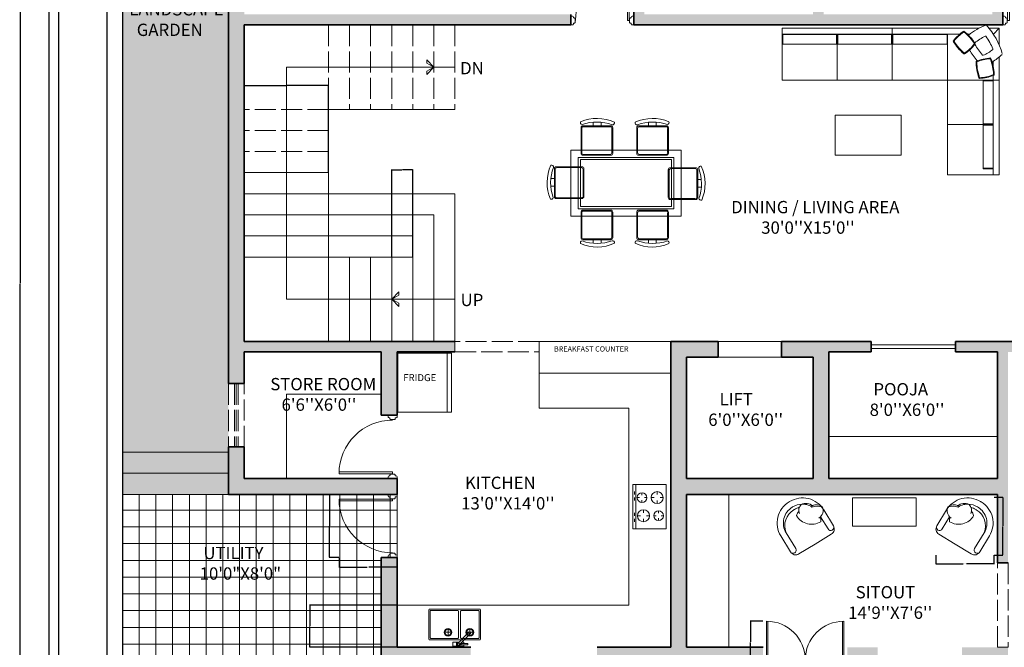
# Model space of a CAD drawing. Units: inches. Extents: x 84 to 1044, y -280 to 906.
# Tile 49 of 105: x 84 to 645, y 160 to 517. Entities that reach past the tile are written whole.
import ezdxf

# ---------------------------------------------------------------- set-up
doc = ezdxf.new("R2010")
doc.units = ezdxf.units.IN
doc.linetypes.add('ACAD_ISO02W100', pattern=[15, 12, -3])
for name, color, linetype, lineweight in [('00 FURNITURE', 15, 'Continuous', 15), ('A-ANNO-DIMS', 2, 'Continuous', 18), ('A-ANNO-SYMB', 7, 'Continuous', 15), ('A-ANNO-TEXT', 7, 'Continuous', 13), ('A-ANNO-TTLB', 7, 'Continuous', 25), ('A-AREA-IDEN', 7, 'Continuous', 13), ('A-DOOR', 4, 'Continuous', 18), ('A-EQPM', 8, 'Continuous', 15), ('A-FLOR-CASE', 8, 'Continuous', 18), ('A-FLOR-FIXT', 9, 'Continuous', 15), ('A-FLOR-STRS-OVHD', 144, 'ACAD_ISO02W100', 13), ('A-FURN', 8, 'Continuous', 15), ('A-GLAZ-HIGH', 160, 'ACAD_ISO02W100', 13), ('A-STAIRCASE', 144, 'Continuous', 18), ('A-WALL-OVHD', 8, 'ACAD_ISO02W100', 13), ('C-PROP', 7, 'Continuous', 25), ('L-HRDS', 32, 'Continuous', 18), ('WALL', 250, 'Continuous', 35), ('WINDOW', 160, 'Continuous', 13)]:
    doc.layers.add(name, color=color, linetype=linetype, lineweight=lineweight)
for name, color, linetype, lineweight, true_color in [('A-FLOR-PATT', 251, 'Continuous', 9, 0x705861), ('A-FLOR-STRS-PATT', 35, 'Continuous', 9, 0x947764), ('A-WALL-PATT', 251, 'Continuous', 9, 0x636466), ('L-PLNT-PATT', 9, 'Continuous', 9, 0xafd9aa)]:
    doc.layers.add(name, color=color, linetype=linetype, lineweight=lineweight, true_color=true_color)
doc.styles.add('1-100DIM', font='txt', dxfattribs={"height": 0.3})
doc.styles.get("Standard").update_dxf_attribs({"font": 'arial.ttf'})
doc.dimstyles.get("Standard").update_dxf_attribs({"dimtxt": 0.18, "dimasz": 0.18, "dimexe": 0.18, "dimexo": 0.0625, "dimgap": 0.09, "dimtad": 0, "dimtih": 1, "dimtoh": 1, "dimdec": 4, "dimzin": 0, "dimdsep": 46, "dimtxsty": 'Standard', "dimcen": 0.09, "dimadec": 0, "dimazin": 0, "dimtfac": 1, "dimtdec": 4, "dimtofl": 0, "dimtmove": 0, "dimatfit": 3, "dimfxl": 1, "dimtolj": 1, "dimtzin": 0, "dimarcsym": 0})

# ---------------------------------------------------------------- blocks, each defined once
blk = doc.blocks.new('PUJA')
at = {"layer": '00 FURNITURE'}
for p, q in [((-1940.35, -16093.35), (-1958.14, -16093.35)), ((-1940.35, -16093.93), (-1958.13, -16093.93)), ((-1941.8, -16091.75), (-1938.89, -16091.75)), ((-1941.8, -16092.33), (-1941.8, -16091.75)), ((-1941.22, -16092.62), (-1941.51, -16092.62)), ((-1940.35, -16093.35), (-1940.35, -16093.93)), ((-1939.18, -16092.62), (-1939.47, -16092.62)), ((-1938.89, -16091.75), (-1938.89, -16092.33)), ((-1940.35, -16128.93), (-1958.14, -16128.93)), ((-1940.35, -16128.35), (-1958.13, -16128.35)), ((-1941.8, -16129.96), (-1941.8, -16130.54)), ((-1941.8, -16130.54), (-1938.89, -16130.54)), ((-1941.22, -16129.66), (-1941.51, -16129.66)), ((-1940.35, -16128.93), (-1940.35, -16128.35)), ((-1939.18, -16129.66), (-1939.47, -16129.66)), ((-1938.89, -16130.54), (-1938.89, -16129.96))]:
    blk.add_line(p, q, dxfattribs=at)
for points in [[(-1939.47, -16092.62), (-1939.47, -16092.91, -0.414214), (-1939.76, -16093.21), (-1940.93, -16093.21, -0.414214), (-1941.22, -16092.91), (-1941.22, -16092.62)], [(-1939.47, -16129.66), (-1939.47, -16129.37, 0.414214), (-1939.76, -16129.08), (-1940.93, -16129.08, 0.414214), (-1941.22, -16129.37), (-1941.22, -16129.66)]]:
    blk.add_lwpolyline(points, format="xyb", dxfattribs=at)
for centre, radius, start, end in [((-1940.35, -16093.35), 17.79, 180, 270), ((-1941.51, -16092.33), 0.292, 180, 270), ((-1939.18, -16092.33), 0.292, 270, 0), ((-1940.35, -16128.93), 17.79, 90, 180), ((-1941.51, -16129.96), 0.292, 90, 180), ((-1939.18, -16129.96), 0.292, 0, 90)]:
    blk.add_arc(centre, radius, start, end, dxfattribs=at)
blk = doc.blocks.new('DDD')
at = {"layer": '00 FURNITURE'}
for p, q in [((-12579.77, -15859.53), (-12579.77, -15829.05)), ((-12578.77, -15859.53), (-12578.77, -15829.03)), ((-12612.02, -15857.03), (-12612.02, -15862.03)), ((-12611.02, -15857.03), (-12612.02, -15857.03)), ((-12610.52, -15858.03), (-12610.52, -15857.53)), ((-12577.52, -15858.03), (-12577.52, -15857.53)), ((-12577.02, -15857.03), (-12576.02, -15857.03)), ((-12576.02, -15857.03), (-12576.02, -15862.03)), ((-12612.02, -15862.03), (-12611.02, -15862.03)), ((-12610.52, -15861.53), (-12610.52, -15861.03)), ((-12578.77, -15859.53), (-12579.77, -15859.53)), ((-12577.52, -15861.53), (-12577.52, -15861.03)), ((-12576.02, -15862.03), (-12577.02, -15862.03))]:
    blk.add_line(p, q, dxfattribs=at)
for points in [[(-12610.52, -15861.03), (-12610.02, -15861.03, 0.414214), (-12609.52, -15860.53), (-12609.52, -15858.53, 0.414214), (-12610.02, -15858.03), (-12610.52, -15858.03)], [(-12577.52, -15861.03), (-12578.02, -15861.03, -0.414214), (-12578.52, -15860.53), (-12578.52, -15858.53, -0.414214), (-12578.02, -15858.03), (-12577.52, -15858.03)]]:
    blk.add_lwpolyline(points, format="xyb", dxfattribs=at)
for centre, radius, start, end in [((-12578.77, -15859.53), 30.5, 90, 180), ((-12611.02, -15857.53), 0.5, 0, 90), ((-12577.02, -15857.53), 0.5, 90, 180), ((-12611.02, -15861.53), 0.5, 270, 0), ((-12577.02, -15861.53), 0.5, 180, 270)]:
    blk.add_arc(centre, radius, start, end, dxfattribs=at)
blk = doc.blocks.new('CHAIR-LOUNGE')
for points in [[(10.9, 6.11), (20.11, 0.51, 0.414214), (24.96, 1.7), (30.46, 10.75, 0.414214), (25.72, 30.16), (25.57, 30.25), (25.42, 30.34, 0.414214), (6.01, 25.61), (0.51, 16.55, 0.414214), (1.69, 11.7), (10.9, 6.11)], [(8.7, 20.85, -0.356772), (6.69, 27.28, -0.249542), (12.51, 28.04, 9.61688)], [(6.69, 27.28, -0.14773), (12.68, 27.2, -0.213343), (18.88, 28.63, -0.178662)], [(12.19, 27.77, -0.306663), (18.88, 28.63, -0.30633), (19.83, 23.56, 0.872847)], [(18.37, 28.86, -0.130591), (23.59, 27.33), (23.74, 27.24)], [(8, 21.4, 0.165541), (7.72, 18.84, 0.425989), (21.45, 22.34, 0.121523), (20.16, 24.75, -7.115464)], [(19.9, 27.06, -0.072384), (22.67, 25.82), (22.82, 25.73)], [(27.44, 12.59, 0.372719), (22.97, 25.63), (22.82, 25.73)], [(27.44, 12.59, 0.414214), (23.89, 27.14), (23.74, 27.24)], [(7.74, 21.66), (3.53, 14.72, -0.414214), (1.1, 14.13), (1.1, 14.13, -0.414214), (0.51, 16.55)], [(27.44, 12.59), (21.94, 3.53, 0.414214), (22.53, 1.11), (22.53, 1.11, 0.414214), (24.96, 1.7)]]:
    blk.add_lwpolyline(points, format="xyb")
blk = doc.blocks.new('WIN-HIGH-36IN')
for p, q in [((3.5, 36), (3.5, 0)), ((4.5, 36), (4.5, 0)), ((5.5, 36), (5.5, 0))]:
    blk.add_line(p, q)
blk.add_lwpolyline([(0, 0), (9, 0), (9, 36), (0, 36)], close=True)
blk = doc.blocks.new('STAIR-DIRECTION-HEAD')
for p, q in [((0, 4.1), (4.1, 8.21)), ((4.1, 6.33), (0, 4.1)), ((4.1, 8.21), (4.1, 6.33)), ((0, 4.1), (4.1, -0.01)), ((4.1, 1.87), (0, 4.1)), ((4.1, -0.01), (4.1, 1.87))]:
    blk.add_line(p, q)
blk = doc.blocks.new('*D38')
at = {"layer": 'A-ANNO-DIMS', "color": 0, "lineweight": -2, "transparency": 16777216}
for p, q in [((266.12, 247.12), (260.6, 247.12)), ((260.78, 246.94), (260.78, 229.3)), ((260.78, 211.3), (260.78, 228.94)), ((266.12, 211.12), (260.6, 211.12))]:
    blk.add_line(p, q, dxfattribs=at)
at = {"layer": 'A-ANNO-DIMS', "color": 0, "transparency": 16777216}
for points in [[(260.75, 246.94), (260.81, 246.94), (260.78, 247.12)], [(260.75, 211.3), (260.81, 211.3), (260.78, 211.12)]]:
    blk.add_solid(points, dxfattribs=at)
at = {"layer": 'Defpoints', "color": 0, "transparency": 16777216}
for p in [(260.78, 247.12), (266.18, 247.12), (266.18, 211.12)]:
    blk.add_point(p, dxfattribs=at)
at = {"layer": 'A-ANNO-DIMS', "color": 0, "transparency": 16777216, "insert": (260.78, 229.12), "char_height": 0.18, "attachment_point": 5}
blk.add_mtext('\\A1;DOOR 36 TYP.', dxfattribs=at)
blk = doc.blocks.new('*D39')
at = {"layer": 'A-ANNO-DIMS', "color": 0, "lineweight": -2, "transparency": 16777216}
for p, q in [((266.18, 211.06), (266.18, 205.54)), ((299.18, 211.06), (299.18, 205.54)), ((266.36, 205.72), (282.15, 205.72)), ((299, 205.72), (283.21, 205.72))]:
    blk.add_line(p, q, dxfattribs=at)
at = {"layer": 'A-ANNO-DIMS', "color": 0, "transparency": 16777216}
for points in [[(266.36, 205.75), (266.36, 205.69), (266.18, 205.72)], [(299, 205.75), (299, 205.69), (299.18, 205.72)]]:
    blk.add_solid(points, dxfattribs=at)
at = {"layer": 'Defpoints', "color": 0, "transparency": 16777216}
for p in [(266.18, 211.12), (299.18, 211.12), (266.18, 205.72)]:
    blk.add_point(p, dxfattribs=at)
at = {"layer": 'A-ANNO-DIMS', "color": 0, "transparency": 16777216, "insert": (282.68, 205.72), "char_height": 0.18, "attachment_point": 5}
blk.add_mtext('\\A1;33 TYP.', dxfattribs=at)
blk = doc.blocks.new('*D43')
at = {"layer": 'A-ANNO-DIMS', "color": 0, "lineweight": -2, "transparency": 16777216}
for p, q in [((507.51, 174.94), (500.19, 174.94)), ((500.37, 174.76), (500.37, 163.21)), ((500.37, 151.3), (500.37, 162.85)), ((507.51, 151.12), (500.19, 151.12))]:
    blk.add_line(p, q, dxfattribs=at)
at = {"layer": 'A-ANNO-DIMS', "color": 0, "transparency": 16777216}
for points in [[(500.34, 174.76), (500.4, 174.76), (500.37, 174.94)], [(500.34, 151.3), (500.4, 151.3), (500.37, 151.12)]]:
    blk.add_solid(points, dxfattribs=at)
at = {"layer": 'Defpoints', "color": 0, "transparency": 16777216}
for p in [(507.57, 174.94), (500.37, 151.12), (507.57, 151.12)]:
    blk.add_point(p, dxfattribs=at)
at = {"layer": 'A-ANNO-DIMS', "color": 0, "transparency": 16777216, "insert": (500.37, 163.03), "char_height": 0.18, "attachment_point": 5}
blk.add_mtext('\\A1;24', dxfattribs=at)
blk = doc.blocks.new('*D58')
at = {"layer": 'A-ANNO-DIMS', "color": 0, "lineweight": -2, "transparency": 16777216}
for p, q in [((605.9, 212.52), (605.9, 207.43)), ((606.08, 207.61), (621.5, 207.61)), ((638.84, 207.61), (623.41, 207.61)), ((639.02, 212.52), (639.02, 207.43))]:
    blk.add_line(p, q, dxfattribs=at)
at = {"layer": 'A-ANNO-DIMS', "color": 0, "transparency": 16777216}
for points in [[(606.08, 207.64), (606.08, 207.58), (605.9, 207.61)], [(638.84, 207.64), (638.84, 207.58), (639.02, 207.61)]]:
    blk.add_solid(points, dxfattribs=at)
at = {"layer": 'Defpoints', "color": 0, "transparency": 16777216}
for p in [(605.9, 212.58), (639.02, 212.58), (639.02, 207.61)]:
    blk.add_point(p, dxfattribs=at)
at = {"layer": 'A-ANNO-DIMS', "color": 0, "transparency": 16777216, "insert": (622.46, 207.61), "char_height": 0.18, "attachment_point": 5}
blk.add_mtext('\\A1;CHAIR 33 TYP.', dxfattribs=at)
blk = doc.blocks.new('*D59')
at = {"layer": 'A-ANNO-DIMS', "color": 0, "lineweight": -2, "transparency": 16777216}
for p, q in [((639.08, 245.58), (644.17, 245.58)), ((643.99, 245.4), (643.99, 229.26)), ((643.99, 212.76), (643.99, 228.9)), ((639.08, 212.58), (644.17, 212.58))]:
    blk.add_line(p, q, dxfattribs=at)
at = {"layer": 'A-ANNO-DIMS', "color": 0, "transparency": 16777216}
for points in [[(643.96, 245.4), (644.02, 245.4), (643.99, 245.58)], [(643.96, 212.76), (644.02, 212.76), (643.99, 212.58)]]:
    blk.add_solid(points, dxfattribs=at)
at = {"layer": 'Defpoints', "color": 0, "transparency": 16777216}
for p in [(639.02, 245.58), (643.99, 245.58), (639.02, 212.58)]:
    blk.add_point(p, dxfattribs=at)
at = {"layer": 'A-ANNO-DIMS', "color": 0, "transparency": 16777216, "insert": (643.99, 229.08), "char_height": 0.18, "attachment_point": 5}
blk.add_mtext('\\A1;33 TYP.', dxfattribs=at)
blk = doc.blocks.new('*D61')
at = {"layer": 'A-ANNO-DIMS', "color": 0, "lineweight": -2, "transparency": 16777216}
for p, q in [((134.12, 856.12), (84.4, 856.12)), ((84.58, 855.94), (84.58, 367.3)), ((84.58, -121.7), (84.58, 366.94)), ((134.12, -121.88), (84.4, -121.88))]:
    blk.add_line(p, q, dxfattribs=at)
at = {"layer": 'A-ANNO-DIMS', "color": 0, "transparency": 16777216}
for points in [[(84.55, 855.94), (84.61, 855.94), (84.58, 856.12)], [(84.55, -121.7), (84.61, -121.7), (84.58, -121.88)]]:
    blk.add_solid(points, dxfattribs=at)
at = {"layer": 'Defpoints', "color": 0, "transparency": 16777216}
for p in [(84.58, 856.12), (134.18, 856.12), (134.18, -121.88)]:
    blk.add_point(p, dxfattribs=at)
at = {"layer": 'A-ANNO-DIMS', "color": 0, "transparency": 16777216, "insert": (84.58, 367.12), "char_height": 0.18, "attachment_point": 5}
blk.add_mtext('\\A1;978', dxfattribs=at)
blk = doc.blocks.new('*D62')
at = {"layer": 'A-ANNO-DIMS', "color": 0, "lineweight": -2, "transparency": 16777216}
for p, q in [((203.18, 709.18), (203.18, 905.9)), ((203.36, 905.72), (549.23, 905.72)), ((895.89, 905.72), (550.02, 905.72)), ((896.07, 400.18), (896.07, 905.9))]:
    blk.add_line(p, q, dxfattribs=at)
at = {"layer": 'A-ANNO-DIMS', "color": 0, "transparency": 16777216}
for points in [[(203.36, 905.75), (203.36, 905.69), (203.18, 905.72)], [(895.89, 905.75), (895.89, 905.69), (896.07, 905.72)]]:
    blk.add_solid(points, dxfattribs=at)
at = {"layer": 'Defpoints', "color": 0, "transparency": 16777216}
for p in [(896.07, 905.72), (203.18, 709.12), (896.07, 400.12)]:
    blk.add_point(p, dxfattribs=at)
at = {"layer": 'A-ANNO-DIMS', "color": 0, "transparency": 16777216, "insert": (549.63, 905.72), "char_height": 0.18, "attachment_point": 5}
blk.add_mtext('\\A1;692.9', dxfattribs=at)
blk = doc.blocks.new('*D71')
at = {"layer": 'A-ANNO-DIMS', "color": 0, "lineweight": -2, "transparency": 16777216}
for p, q in [((212.18, 430.18), (212.18, 479.9)), ((212.36, 479.72), (235.96, 479.72)), ((260, 479.72), (236.4, 479.72)), ((260.18, 430.18), (260.18, 479.9))]:
    blk.add_line(p, q, dxfattribs=at)
at = {"layer": 'A-ANNO-DIMS', "color": 0, "transparency": 16777216}
for points in [[(212.36, 479.75), (212.36, 479.69), (212.18, 479.72)], [(260, 479.75), (260, 479.69), (260.18, 479.72)]]:
    blk.add_solid(points, dxfattribs=at)
at = {"layer": 'Defpoints', "color": 0, "transparency": 16777216}
for p in [(260.18, 479.72), (212.18, 430.12), (260.18, 430.12)]:
    blk.add_point(p, dxfattribs=at)
at = {"layer": 'A-ANNO-DIMS', "color": 0, "transparency": 16777216, "insert": (236.18, 479.72), "char_height": 0.18, "attachment_point": 5}
blk.add_mtext('\\A1;48', dxfattribs=at)
blk = doc.blocks.new('*D72')
at = {"layer": 'A-ANNO-DIMS', "color": 0, "lineweight": -2, "transparency": 16777216}
for p, q in [((296.18, 382.18), (296.18, 431.9)), ((296.36, 431.72), (301.97, 431.72)), ((308, 431.72), (302.39, 431.72)), ((308.18, 382.18), (308.18, 431.9))]:
    blk.add_line(p, q, dxfattribs=at)
at = {"layer": 'A-ANNO-DIMS', "color": 0, "transparency": 16777216}
for points in [[(296.36, 431.75), (296.36, 431.69), (296.18, 431.72)], [(308, 431.75), (308, 431.69), (308.18, 431.72)]]:
    blk.add_solid(points, dxfattribs=at)
at = {"layer": 'Defpoints', "color": 0, "transparency": 16777216}
for p in [(308.18, 431.72), (296.18, 382.12), (308.18, 382.12)]:
    blk.add_point(p, dxfattribs=at)
at = {"layer": 'A-ANNO-DIMS', "color": 0, "transparency": 16777216, "insert": (302.18, 431.72), "char_height": 0.18, "attachment_point": 5}
blk.add_mtext('\\A1;12', dxfattribs=at)
blk = doc.blocks.new('*D79')
at = {"layer": 'A-ANNO-DIMS', "color": 0, "lineweight": -2, "transparency": 16777216}
for p, q in [((299.12, 184.12), (249.4, 184.12)), ((249.58, 183.94), (249.58, 172.3)), ((249.58, 160.3), (249.58, 171.94)), ((299.12, 160.12), (249.4, 160.12))]:
    blk.add_line(p, q, dxfattribs=at)
at = {"layer": 'A-ANNO-DIMS', "color": 0, "transparency": 16777216}
for points in [[(249.55, 183.94), (249.61, 183.94), (249.58, 184.12)], [(249.55, 160.3), (249.61, 160.3), (249.58, 160.12)]]:
    blk.add_solid(points, dxfattribs=at)
at = {"layer": 'Defpoints', "color": 0, "transparency": 16777216}
for p in [(249.58, 184.12), (299.18, 184.12), (299.18, 160.12)]:
    blk.add_point(p, dxfattribs=at)
at = {"layer": 'A-ANNO-DIMS', "color": 0, "transparency": 16777216, "insert": (249.58, 172.12), "char_height": 0.18, "attachment_point": 5}
blk.add_mtext('\\A1;24', dxfattribs=at)

msp = doc.modelspace()

# ---------------------------------------------------------------- hatches: boundary and pattern name
at = {"layer": 'A-FLOR-PATT', "transparency": 33554597}
h = msp.add_hatch(dxfattribs=at)
h.set_pattern_fill('ANSI37', color=256, scale=3, angle=45)
h.paths.add_polyline_path([(290.179, 211.12), (299.179, 211.12), (299.179, 247.12), (203.179, 247.12), (143.179, 247.12), (143.179, 151.12), (203.179, 151.12), (203.179, 155.12), (290.179, 155.12)])
at = {"layer": 'A-FLOR-STRS-PATT', "transparency": 33554567}
h = msp.add_hatch(color=256, dxfattribs=at)
h.dxf.hatch_style = 1
h.paths.add_polyline_path([(650.074, 91.12), (638.074, 91.12), (638.074, 67.12), (455.074, 67.12), (455.074, 55.12), (650.074, 55.12)], flags=17)
h.paths.add_polyline_path([(662.074, 91.12), (650.074, 91.12), (650.074, 55.12), (455.074, 55.12), (455.074, 43.12), (662.074, 43.12)])
h.paths.add_polyline_path([(674.074, 91.12), (671.074, 91.12), (662.074, 91.12), (662.074, 43.12), (455.074, 43.12), (455.074, 31.12), (674.074, 31.12)])
h.paths.add_polyline_path([(227.179, 151.12), (203.179, 151.12), (143.179, 151.12), (143.179, 139.12), (227.179, 139.12)])
h.paths.add_polyline_path([(227.179, 139.12), (143.179, 139.12), (143.179, 127.12), (227.179, 127.12)])
h.paths.add_polyline_path([(203.179, 271.12), (143.179, 271.12), (143.179, 259.12), (203.179, 259.12)])
h.paths.add_polyline_path([(203.179, 259.12), (143.179, 259.12), (143.179, 247.12), (203.179, 247.12)])
h.paths.add_polyline_path([(203.179, 769.12), (143.179, 769.12), (143.179, 757.12), (203.179, 757.12)])
h.paths.add_polyline_path([(203.179, 757.12), (143.179, 757.12), (143.179, 745.12), (203.179, 745.12)])
h.paths.add_polyline_path([(434.074, 847.12), (422.074, 847.12), (422.074, 769.12), (434.074, 769.12)])
h.paths.add_polyline_path([(422.074, 847.12), (410.074, 847.12), (410.074, 769.12), (422.074, 769.12)])
at = {"layer": 'A-WALL-PATT', "transparency": 33554597}
h = msp.add_hatch(color=256, dxfattribs=at)
h.dxf.hatch_style = 1
h.paths.add_polyline_path([(671.074, 100.12), (647.074, 100.12), (647.074, 160.12), (641.074, 160.12), (620.824, 160.12), (620.824, 151.12), (638.074, 151.12), (638.074, 91.12), (671.074, 91.12)])
h.paths.add_polyline_path([(791.074, 100.12), (743.074, 100.12), (743.074, 91.12), (791.074, 91.12)])
h.paths.add_polyline_path([(896.074, 346.12), (887.074, 346.12), (887.074, 334.12), (870.955, 334.12), (833.074, 334.12), (804.574, 334.12), (804.574, 328.12), (887.074, 328.12), (887.074, 100.12), (863.074, 100.12), (863.074, 91.12), (896.074, 91.12)])
h.paths.add_polyline_path([(507.574, 154.729), (507.574, 160.12), (464.074, 160.12), (464.074, 247.12), (641.074, 247.12), (641.074, 208.12), (647.074, 208.12), (647.074, 328.12), (659.074, 328.12), (659.074, 334.12), (617.074, 334.12), (617.074, 328.12), (641.074, 328.12), (641.074, 256.12), (545.074, 256.12), (545.074, 328.12), (569.074, 328.12), (569.074, 334.12), (518.074, 334.12), (518.074, 325.12), (536.074, 325.12), (536.074, 256.12), (464.074, 256.12), (464.074, 325.12), (482.074, 325.12), (482.074, 334.12), (455.074, 334.12), (455.074, 160.12), (413.127, 160.12), (413.127, 151.12), (455.074, 151.12), (455.074, 91.12), (464.074, 91.12), (464.074, 151.12), (507.574, 151.12)])
h.paths.add_polyline_path([(572.824, 160.12), (555.574, 160.12), (555.574, 151.12), (572.824, 151.12)], flags=17)
h.paths.add_polyline_path([(341.127, 160.12), (299.179, 160.12), (299.179, 211.12), (294.179, 211.12), (290.179, 211.12), (290.179, 151.12), (341.127, 151.12)])
h.paths.add_polyline_path([(299.179, 256.12), (212.179, 256.12), (212.179, 274.12), (203.179, 274.12), (203.179, 247.12), (299.179, 247.12)])
h.paths.add_polyline_path([(212.179, 514.12), (398.074, 514.12), (398.074, 519.12), (398.074, 520.12), (212.179, 520.12), (212.179, 574.12), (203.179, 574.12), (203.179, 310.12), (212.179, 310.12), (212.179, 328.12), (290.179, 328.12), (290.179, 292.12), (299.179, 292.12), (299.179, 328.12), (332.179, 328.12), (332.179, 334.12), (212.179, 334.12)])
h.paths.add_polyline_path([(287.127, 709.12), (203.179, 709.12), (203.179, 646.12), (212.179, 646.12), (212.179, 700.12), (287.127, 700.12)])
h.paths.add_polyline_path([(470.074, 709.12), (359.127, 709.12), (359.127, 700.12), (434.074, 700.12), (434.074, 574.12), (440.074, 574.12), (440.074, 622.12), (464.074, 622.12), (464.074, 628.12), (440.074, 628.12), (440.074, 700.12), (470.074, 700.12)])
h.paths.add_polyline_path([(572.074, 709.12), (506.074, 709.12), (506.074, 700.12), (536.074, 700.12), (536.074, 628.12), (494.074, 628.12), (494.074, 622.12), (536.074, 622.12), (536.074, 520.12), (440.074, 520.12), (440.074, 544.12), (434.074, 544.12), (434.074, 514.12), (644.074, 514.12), (644.074, 519.12), (644.074, 544.12), (638.074, 544.12), (638.074, 520.12), (542.074, 520.12), (542.074, 622.12), (584.074, 622.12), (584.074, 628.12), (542.074, 628.12), (542.074, 700.12), (572.074, 700.12)])
h.paths.add_polyline_path([(698.074, 709.12), (608.074, 709.12), (608.074, 700.12), (638.074, 700.12), (638.074, 628.12), (614.074, 628.12), (614.074, 622.12), (638.074, 622.12), (638.074, 574.12), (644.074, 574.12), (644.074, 700.12), (698.074, 700.12)])
h.paths.add_polyline_path([(833.074, 709.12), (770.074, 709.12), (770.074, 700.12), (824.074, 700.12), (824.074, 646.12), (833.074, 646.12)])
h.paths.add_polyline_path([(833.074, 574.12), (824.074, 574.12), (824.074, 520.12), (791.244, 520.12), (712.904, 520.12), (680.074, 520.12), (680.074, 514.12), (695.074, 514.12), (695.074, 491.62), (704.074, 491.62), (704.074, 511.12), (833.074, 511.12)])
h.paths.add_polyline_path([(704.074, 419.62), (695.074, 419.62), (695.074, 370.12), (704.074, 370.12)])
h.paths.add_polyline_path([(896.074, 400.12), (833.074, 400.12), (833.074, 364.12), (839.074, 364.12), (839.074, 394.12), (887.074, 394.12), (887.074, 382.12), (896.074, 382.12)])
h.paths.add_polyline_path([(732.574, 334.12), (695.074, 334.12), (695.074, 328.12), (732.574, 328.12)])
at = {"layer": 'L-PLNT-PATT', "transparency": 33554597}
h = msp.add_hatch(color=256, dxfattribs=at)
h.dxf.hatch_style = 1
h.paths.add_polyline_path([(434.074, 769.12), (386.074, 769.12), (386.074, 709.12), (434.074, 709.12)])
h.paths.add_polyline_path([(896.074, 847.12), (434.074, 847.12), (434.074, 769.12), (434.074, 709.12), (470.074, 709.12), (506.074, 709.12), (572.074, 709.12), (608.074, 709.12), (698.074, 709.12), (770.074, 709.12), (833.074, 709.12), (896.074, 709.12)])
h.paths.add_polyline_path([(983.074, 847.12), (896.074, 847.12), (896.074, 709.12), (896.074, 547.12), (932.074, 547.12), (983.074, 547.12)])
h.paths.add_polyline_path([(983.074, 547.12), (932.074, 547.12), (932.074, 265.12), (983.074, 265.12)])
h.paths.add_polyline_path([(203.179, 646.12), (203.179, 709.12), (203.179, 745.12), (143.179, 745.12), (143.179, 271.12), (203.179, 271.12), (203.179, 274.12), (203.179, 310.12), (203.179, 574.12)])

# ---------------------------------------------------------------- linework, layer by layer
at = {"layer": 'A-ANNO-SYMB'}
msp.add_lwpolyline([(332.179, 358.12), (236.179, 358.12), (236.179, 490.12), (332.179, 490.12)], dxfattribs=at)
at = {"layer": 'A-ANNO-TTLB'}
for points in [[(101.1, 905.916), (1027.308, 905.916), (1027.308, -279.764), (101.1, -279.764)], [(106.576, 900.439), (1021.832, 900.439), (1021.832, -274.288), (106.576, -274.288)]]:
    msp.add_lwpolyline(points, close=True, dxfattribs=at)
at = {"layer": 'A-DOOR'}
msp.add_line((299.179, 247.12), (299.179, 211.12), dxfattribs=at)
at = {"layer": 'A-EQPM'}
for p, q in [((482.074, 334.12), (518.074, 334.12)), ((482.074, 325.12), (518.074, 325.12)), ((433.49, 252.811), (433.49, 227.429)), ((452.402, 252.811), (433.49, 252.811)), ((435.209, 252.811), (435.209, 227.429)), ((452.402, 227.429), (452.402, 252.811)), ((434.35, 248.716), (434.35, 246.997)), ((438.648, 248.028), (438.648, 246.653)), ((447.244, 248.716), (447.244, 246.997)), ((434.35, 245.278), (434.35, 243.558)), ((435.897, 245.278), (437.272, 245.278)), ((438.648, 242.527), (438.648, 243.902)), ((441.399, 245.278), (440.023, 245.278)), ((443.805, 245.278), (445.525, 245.278)), ((447.244, 241.839), (447.244, 243.558)), ((450.682, 245.278), (448.963, 245.278)), ((434.35, 236.682), (434.35, 234.962)), ((439.507, 238.401), (439.507, 236.682)), ((448.104, 237.713), (448.104, 236.338)), ((434.35, 233.243), (434.35, 231.524)), ((436.069, 234.962), (437.788, 234.962)), ((439.507, 231.524), (439.507, 233.243)), ((442.946, 234.962), (441.227, 234.962)), ((445.353, 234.962), (446.728, 234.962)), ((448.104, 232.212), (448.104, 233.587)), ((450.854, 234.962), (449.479, 234.962)), ((433.49, 227.429), (452.402, 227.429))]:
    msp.add_line(p, q, dxfattribs=at)
for points in [[(299.707, 327.424), (327.675, 327.424), (327.675, 293.944), (299.707, 293.944)], [(327.675, 327.424), (330.111, 327.424), (330.111, 293.944), (327.675, 293.944)]]:
    msp.add_lwpolyline(points, close=True, dxfattribs=at)
for centre, major_axis, start_param, end_param in [((438.648, 245.278), (1.945, 1.945), -0.8050353, 5.47815), ((447.244, 245.278), (3.438, -0.065), 3.1674886, 9.4506739), ((439.507, 234.962), (3.438, -0.027), 3.1547976, 9.4379829), ((448.104, 234.962), (1.945, 1.945), -0.8033148, 5.4798705)]:
    msp.add_ellipse(centre, major_axis=major_axis, ratio=1, start_param=start_param, end_param=end_param, dxfattribs=at)
at = {"layer": 'A-FLOR-CASE'}
for p, q in [((455.074, 334.12), (380.179, 334.12)), ((380.179, 334.12), (380.179, 296.12)), ((455.074, 316.12), (380.179, 316.12)), ((236.179, 304.12), (236.179, 256.12)), ((290.179, 304.12), (236.179, 304.12)), ((431.074, 296.12), (380.179, 296.12)), ((431.074, 296.12), (431.074, 184.12)), ((641.074, 280.12), (545.074, 280.12)), ((488.074, 247.12), (488.074, 160.12)), ((299.179, 184.12), (431.074, 184.12))]:
    msp.add_line(p, q, dxfattribs=at)
at = {"layer": 'A-FLOR-FIXT'}
for p, q in [((317.284, 181.485), (317.284, 164.72)), ((346.27, 181.876), (317.676, 181.876)), ((318.068, 180.701), (318.068, 165.503)), ((333.736, 181.093), (318.459, 181.093)), ((334.127, 165.503), (334.127, 180.701)), ((346.662, 164.72), (346.662, 181.485)), ((325.959, 168.637), (330.464, 168.637)), ((328.212, 166.385), (328.212, 170.889)), ((338.397, 168.637), (342.901, 168.637)), ((340.329, 168.972), (339.194, 167.781)), ((340.62, 167.518), (339.761, 168.376)), ((341.215, 168.086), (340.329, 168.972)), ((340.649, 166.385), (340.649, 170.889)), ((317.676, 164.328), (346.27, 164.328)), ((318.459, 165.112), (333.736, 165.112)), ((334.413, 163), (331.033, 163)), ((331.033, 163), (331.033, 160.846)), ((333.031, 160.846), (333.031, 163)), ((333.031, 162.608), (334.021, 162.608)), ((333.751, 162.338), (339.194, 167.781)), ((340.024, 166.95), (334.582, 161.507)), ((337.222, 163), (336.075, 163)), ((337.222, 162.295), (337.222, 163)), ((340.024, 166.95), (339.194, 167.781)), ((340.024, 166.95), (341.215, 168.086)), ((331.033, 160.846), (337.222, 160.846)), ((335.185, 161.237), (333.031, 161.237)), ((335.185, 162.11), (335.185, 160.846)), ((335.655, 161.551), (335.655, 162.295)), ((335.655, 162.295), (339.415, 162.295)), ((339.415, 161.551), (335.655, 161.551)), ((337.222, 160.846), (337.222, 161.551)), ((339.415, 162.295), (339.415, 161.551))]:
    msp.add_line(p, q, dxfattribs=at)
msp.add_lwpolyline([(333.736, 181.093), (318.459, 181.093, 0.4142136), (318.068, 180.701), (318.068, 165.503, 0.4142136), (318.459, 165.112), (333.736, 165.112)], format="xyb", dxfattribs=at)
msp.add_lwpolyline([(345.487, 181.093), (335.812, 181.093, 0.4142136), (335.42, 180.701), (335.42, 165.503, 0.4142136), (335.812, 165.112), (345.487, 165.112, 0.4142136), (345.878, 165.503), (345.878, 180.701, 0.4142136)], format="xyb", close=True, dxfattribs=at)
msp.add_lwpolyline([(336.524, 165.112), (337.653, 165.112)], dxfattribs=at)
for centre, radius in [((328.212, 168.637), 2.252), ((328.212, 168.637), 1.763), ((340.649, 168.637), 2.252), ((340.649, 168.637), 1.763), ((334.166, 161.923), 0.685)]:
    msp.add_circle(centre, radius, dxfattribs=at)
for centre, radius, start, end in [((317.676, 181.485), 0.392, 90, 180), ((318.459, 180.701), 0.392, 90, 180), ((333.736, 180.701), 0.392, 0, 90), ((346.27, 181.485), 0.392, 0, 90), ((317.676, 164.72), 0.392, 180, 270), ((318.459, 165.503), 0.392, 180, 270), ((333.736, 165.503), 0.392, 270, 0), ((346.27, 164.72), 0.392, 270, 0), ((334.166, 161.923), 0.588, 135, 315)]:
    msp.add_arc(centre, radius, start, end, dxfattribs=at)
at = {"layer": 'A-FLOR-STRS-OVHD'}
for p, q in [((260.179, 514.12), (260.179, 466.12)), ((272.179, 514.12), (272.179, 466.12)), ((284.179, 514.12), (284.179, 466.12)), ((296.179, 514.12), (296.179, 466.12)), ((308.179, 514.12), (308.179, 466.12)), ((320.179, 514.12), (320.179, 466.12)), ((332.179, 514.12), (332.179, 466.12)), ((260.179, 466.12), (212.179, 466.12)), ((260.179, 454.12), (212.179, 454.12)), ((260.179, 442.12), (212.179, 442.12))]:
    msp.add_line(p, q, dxfattribs=at)
at = {"layer": 'A-FURN'}
for p, q in [((518.39, 512.262), (571.767, 512.262)), ((518.39, 482.763), (518.39, 512.262)), ((630.496, 512.262), (571.767, 512.262)), ((581.128, 512.262), (581.128, 482.763)), ((642.001, 512.262), (636.247, 512.262)), ((638.678, 508.939), (642.001, 512.262)), ((642.001, 502.77), (642.001, 512.262)), ((518.39, 508.89), (571.767, 508.89)), ((549.689, 508.792), (518.53, 508.792)), ((518.53, 508.792), (518.53, 503.173)), ((518.811, 508.792), (518.811, 503.173)), ((549.408, 503.173), (549.408, 508.792)), ((549.689, 503.173), (549.689, 508.792)), ((549.759, 482.763), (549.759, 508.89)), ((549.829, 508.792), (580.707, 508.792)), ((549.829, 503.173), (549.829, 508.792)), ((550.11, 503.173), (550.11, 508.792)), ((571.767, 508.89), (606.884, 508.89)), ((580.707, 508.792), (580.707, 503.173)), ((580.707, 508.792), (580.988, 508.792)), ((580.988, 508.792), (580.988, 503.173)), ((581.259, 508.792), (581.259, 503.201)), ((581.259, 508.792), (581.54, 508.792)), ((612.362, 508.792), (581.54, 508.792)), ((581.54, 508.792), (581.54, 503.201)), ((606.884, 508.89), (619.58, 508.89)), ((612.362, 503.201), (612.362, 508.792)), ((612.503, 508.89), (612.503, 428.796)), ((623.968, 508.89), (625.314, 508.89)), ((549.689, 503.173), (518.53, 503.173)), ((549.829, 503.173), (580.988, 503.173)), ((581.259, 503.201), (612.362, 503.201)), ((638.63, 493.51), (638.63, 490.409)), ((642.001, 491.191), (642.001, 495.931)), ((642.001, 491.191), (642.001, 482.763)), ((518.39, 482.763), (642.001, 482.763)), ((638.56, 482.632), (632.941, 482.632)), ((632.941, 457.573), (632.941, 482.632)), ((638.56, 482.632), (632.941, 482.632)), ((638.56, 482.351), (632.941, 482.351)), ((638.56, 457.573), (638.56, 482.632)), ((638.63, 485.441), (638.63, 482.763)), ((638.63, 482.763), (638.63, 444.837)), ((642.001, 428.796), (642.001, 482.763)), ((612.503, 457.479), (638.63, 457.479)), ((632.941, 457.854), (638.56, 457.854)), ((632.941, 457.573), (638.56, 457.573)), ((632.941, 457.376), (632.941, 432.317)), ((632.941, 457.376), (638.56, 457.376)), ((632.941, 457.095), (638.56, 457.095)), ((638.56, 457.376), (638.56, 432.317)), ((638.63, 444.837), (638.63, 428.796)), ((638.56, 432.598), (632.941, 432.598)), ((638.56, 432.598), (632.941, 432.598)), ((638.56, 432.317), (632.941, 432.317)), ((638.56, 432.317), (632.941, 432.317)), ((638.56, 432.317), (638.56, 428.796))]:
    msp.add_line(p, q, dxfattribs=at)
for points in [[(404.576, 457.46, -0.1758093), (421.654, 457.331, 0.5783921), (422.947, 458.754, 0.2145244), (403.67, 459.012, 0.552014), (404.576, 457.46, -0.065079)], [(436.031, 457.331, -0.5783921), (434.737, 458.754, -0.2145244), (454.015, 459.012, -0.552014), (453.109, 457.46, 0.1758093), (436.031, 457.331)], [(405.074, 456.775, 0.4142136), (403.965, 455.666), (403.965, 441.088, 0.4142136), (405.074, 439.979), (420.929, 439.979, 0.4142136), (422.038, 441.088), (422.038, 455.666, 0.4142136), (420.929, 456.775), (405.074, 456.775)], [(415.36, 456.775), (415.36, 458.78, -0.0647586)], [(436.756, 456.775), (452.61, 456.775, -0.4142136), (453.72, 455.666), (453.72, 441.088, -0.4142136), (452.61, 439.979), (436.756, 439.979, -0.4142136), (435.647, 441.088), (435.647, 455.666, -0.4142136), (436.756, 456.775)], [(442.325, 456.775), (442.325, 458.78, 0.0647586)], [(388.09, 415.992, -0.1758092), (388.22, 433.07, 0.5783921), (386.797, 434.364, 0.2145244), (386.538, 415.087, 0.552014), (388.09, 415.992, -0.065079)], [(388.776, 416.491, 0.4142136), (389.885, 415.382), (404.463, 415.382, 0.4142136), (405.572, 416.491), (405.572, 432.346, 0.4142136), (404.463, 433.455), (389.885, 433.455, 0.4142136), (388.776, 432.346), (388.776, 416.491)], [(470.42, 415.948, -0.4142136), (469.311, 414.839), (454.733, 414.839, -0.4142136), (453.624, 415.948), (453.624, 431.803, -0.4142136), (454.733, 432.912), (469.311, 432.912, -0.4142136), (470.42, 431.803), (470.42, 415.948)], [(470.976, 432.527, -0.5783921), (472.399, 433.821, -0.2145244), (472.657, 414.544, -0.552014), (471.105, 415.449, 0.1758094), (470.976, 432.527)], [(388.776, 426.777), (386.771, 426.777, -0.0647586)], [(470.42, 426.234), (472.425, 426.234, 0.0647586)], [(405.074, 391.972, -0.4142136), (403.965, 393.081), (403.965, 407.659, -0.4142136), (405.074, 408.768), (420.929, 408.768, -0.4142136), (422.038, 407.659), (422.038, 393.081, -0.4142136), (420.929, 391.972), (405.074, 391.972)], [(436.756, 391.972), (452.61, 391.972, 0.4142136), (453.72, 393.081), (453.72, 407.659, 0.4142136), (452.61, 408.768), (436.756, 408.768, 0.4142136), (435.647, 407.659), (435.647, 393.081, 0.4142136), (436.756, 391.972)], [(421.654, 391.416, -0.5783921), (422.947, 389.993, -0.2145244), (403.67, 389.735, -0.552014), (404.576, 391.287, 0.1758092), (421.654, 391.416)], [(415.36, 391.972), (415.36, 389.967, 0.0647586)], [(453.109, 391.287, -0.1758092), (436.031, 391.416, 0.5783921), (434.737, 389.993, 0.2145244), (454.015, 389.735, 0.552014), (453.109, 391.287, -0.065079)], [(442.325, 391.972), (442.325, 389.967, -0.0647586)], [(537.213, 218.808), (528.008, 213.214, -0.4142136), (523.156, 214.398), (517.654, 223.453, -0.4142136), (522.39, 242.861), (522.541, 242.953), (522.692, 243.045, -0.4142136), (542.101, 238.308), (547.603, 229.254, -0.4142136), (546.419, 224.402), (537.213, 218.808)], [(529.746, 241.564, 0.1305915), (524.526, 240.027), (524.375, 239.935)], [(535.919, 240.472, 0.3066635), (529.232, 241.334, 0.30633), (528.288, 236.262, -0.8728472)], [(541.422, 239.982, 0.1477299), (535.435, 239.895, 0.2133428), (529.232, 241.334, 0.1786618)], [(539.409, 233.55, 0.3567724), (541.422, 239.982, 0.2495421), (535.599, 240.735, -9.6168803)], [(520.672, 225.287, -0.4142136), (524.224, 239.843), (524.375, 239.935)], [(520.672, 225.287, -0.3727189), (525.141, 238.334), (525.292, 238.426)], [(528.214, 239.756, 0.0723842), (525.443, 238.518), (525.292, 238.426)], [(540.114, 234.104, -0.1655406), (540.392, 231.543, -0.4259892), (526.664, 235.038, -0.1215233), (527.951, 237.452, 7.1154643)], [(540.368, 234.358), (544.585, 227.42, 0.4142136), (547.011, 226.828), (547.011, 226.828, 0.4142136), (547.603, 229.254)], [(520.672, 225.287), (526.174, 216.232, -0.4142136), (525.582, 213.806), (525.582, 213.806, -0.4142136), (523.156, 214.398)]]:
    msp.add_lwpolyline(points, format="xyb", dxfattribs=at)
for points in [[(586.12, 462.743), (548.667, 462.743), (548.667, 440.099), (586.12, 440.099)], [(460.865, 405.362), (398.163, 405.362), (398.163, 442.982), (460.865, 442.982)], [(456.685, 409.542), (402.344, 409.542), (402.344, 438.802), (456.685, 438.802)], [(455.431, 410.796), (403.598, 410.796), (403.598, 437.548), (455.431, 437.548)], [(558.525, 245.109), (594.768, 245.109), (594.768, 229.01), (558.525, 229.01)]]:
    msp.add_lwpolyline(points, close=True, dxfattribs=at)
for points in [[(405.081, 456.275), (420.429, 456.275, -0.4142136), (421.539, 455.166), (421.539, 441.587, -0.4142136), (420.429, 440.478), (405.081, 440.478, -0.5120695), (404.465, 441.587), (404.465, 455.166, -0.5120695)], [(452.604, 456.275), (437.255, 456.275, 0.4142136), (436.146, 455.166), (436.146, 441.587, 0.4142136), (437.255, 440.478), (452.604, 440.478, 0.5120695), (453.22, 441.587), (453.22, 455.166, 0.5120695)], [(389.276, 416.498), (389.276, 431.846, -0.4142136), (390.385, 432.955), (403.963, 432.955, -0.4142136), (405.073, 431.846), (405.073, 416.498, -0.5120695), (403.963, 415.882), (390.385, 415.882, -0.5120695)], [(469.92, 415.955), (469.92, 431.303, 0.4142136), (468.811, 432.412), (455.232, 432.412, 0.4142136), (454.123, 431.303), (454.123, 415.955, 0.5120695), (455.232, 415.339), (468.811, 415.339, 0.5120695)], [(405.081, 392.472), (420.429, 392.472, 0.4142136), (421.539, 393.581), (421.539, 407.16, 0.4142136), (420.429, 408.269), (405.081, 408.269, 0.5120695), (404.465, 407.16), (404.465, 393.581, 0.5120695)], [(452.604, 392.472), (437.255, 392.472, -0.4142136), (436.146, 393.581), (436.146, 407.16, -0.4142136), (437.255, 408.269), (452.604, 408.269, -0.5120695), (453.22, 407.16), (453.22, 393.581, -0.5120695)]]:
    msp.add_lwpolyline(points, format="xyb", close=True, dxfattribs=at)
for points in [[(410.922, 458.817), (410.922, 456.775)], [(446.763, 458.817), (446.763, 456.775)], [(642.001, 428.796), (612.503, 428.796)], [(386.734, 422.339), (388.776, 422.339)], [(472.462, 421.796), (470.42, 421.796)], [(410.922, 389.93), (410.922, 391.972)], [(446.763, 389.93), (446.763, 391.972)]]:
    msp.add_lwpolyline(points, dxfattribs=at)
for centre, radius, start, end in [((640.253, 484.807), 31.739, 125.43825, 140.59871), ((606.794, 490.563), 25.117, 31.4121, 53.16864), ((606.794, 490.563), 25.117, 31.4121, 53.16864), ((647.671, 480.194), 36.378, 111.49081, 129.40892), ((604.862, 486.745), 40.449, 15.89036, 42.2347), ((643.121, 521.973), 32.25, 211.85241, 228.71855), ((616.7, 504.889), 0.393, 139.54841, 212.88585), ((643.121, 521.973), 31.857, 212.88585, 228.71855), ((640.253, 484.807), 31.346, 126.5116, 139.54841), ((621.837, 509.685), 0.393, 51.8077, 126.5116), ((606.794, 490.563), 24.723, 31.4121, 51.8077), ((647.671, 480.194), 30.759, 116.23559, 129.57424), ((634.198, 507.532), 0.281, 35.32124, 116.23559), ((604.862, 486.745), 36.235, 22.26714, 35.32124), ((610.475, 516.269), 21.628, 302.52404, 323.64503), ((610.475, 516.269), 22.021, 302.52404, 323.64503), ((662.879, 522.044), 43.768, 210.46449, 220.32231), ((659.815, 520.857), 36.235, 209.19902, 221.27228), ((627.894, 503.449), 0.393, 323.64503, 31.4121), ((624.378, 517.097), 21.939, 292.86049, 309.43227), ((638.135, 500.369), 0.281, 309.43227, 22.26714), ((622.104, 498.033), 0.393, 228.71855, 302.52404), ((640.031, 463.204), 32.281, 95.19604, 110.3565), ((661.59, 494.391), 32.801, 181.6102, 198.47634), ((629.623, 492.915), 0.4, 109.3062, 182.64364), ((640.031, 463.204), 31.881, 96.26939, 109.3062), ((632.792, 497.14), 0.281, 221.27228, 292.86049), ((636.593, 494.497), 0.4, 21.5655, 96.26939), ((613.58, 485.401), 25.145, 1.16989, 21.5655), ((613.58, 485.401), 25.545, 1.16989, 22.92643), ((622.55, 519.453), 30.523, 300.27955, 313.746), ((661.59, 494.391), 32.401, 182.64364, 198.47634), ((630.859, 484.122), 0.4, 198.47634, 272.28183), ((629.983, 506.102), 21.997, 272.28183, 293.40282), ((629.983, 506.102), 22.397, 272.28183, 293.40282), ((638.72, 485.915), 0.4, 293.40282, 1.16989)]:
    msp.add_arc(centre, radius, start, end, dxfattribs=at)
at = {"layer": 'A-STAIRCASE'}
for p, q in [((260.179, 382.12), (260.179, 466.12)), ((260.179, 466.12), (332.179, 466.12)), ((260.179, 430.12), (212.179, 430.12)), ((260.179, 418.12), (212.179, 418.12)), ((332.179, 418.12), (260.179, 418.12)), ((332.179, 382.12), (332.179, 418.12)), ((260.179, 406.12), (212.179, 406.12)), ((320.179, 406.12), (260.179, 406.12)), ((320.179, 382.12), (320.179, 406.12)), ((260.179, 394.12), (212.179, 394.12)), ((308.179, 394.12), (260.179, 394.12)), ((308.179, 382.12), (308.179, 394.12)), ((260.179, 382.12), (212.179, 382.12)), ((260.179, 382.12), (260.179, 334.12)), ((308.179, 382.12), (260.179, 382.12)), ((272.179, 382.12), (272.179, 334.12)), ((284.179, 382.12), (284.179, 334.12)), ((296.179, 382.12), (296.179, 334.12)), ((308.179, 382.12), (308.179, 334.12)), ((320.179, 382.12), (320.179, 334.12)), ((332.179, 382.12), (332.179, 328.12)), ((203.179, 271.12), (143.179, 271.12)), ((143.179, 271.12), (143.179, 247.12)), ((203.179, 259.12), (143.179, 259.12)), ((143.179, 247.12), (143.179, 127.12))]:
    msp.add_line(p, q, dxfattribs=at)
at = {"layer": 'A-WALL-OVHD'}
for points in [[(332.179, 328.12), (380.179, 328.12), (380.179, 334.12), (332.179, 334.12)], [(641.074, 208.12), (647.074, 208.12), (647.074, 160.12), (641.074, 160.12)]]:
    msp.add_lwpolyline(points, close=True, dxfattribs=at)
at = {"layer": 'C-PROP'}
for points in [[(143.179, -121.88), (134.179, -121.88), (134.179, 856.12), (992.074, 856.12), (992.074, -121.88), (624.574, -121.88)], [(143.179, -112.88), (143.179, 847.12), (983.074, 847.12), (983.074, -112.88), (624.574, -112.88)]]:
    msp.add_lwpolyline(points, dxfattribs=at)
at = {"layer": 'L-HRDS'}
msp.add_line((203.179, 247.12), (143.179, 247.12), dxfattribs=at)
at = {"layer": 'WALL'}
for p, q in [((203.179, 574.12), (203.179, 310.12)), ((434.074, 514.12), (434.074, 544.12)), ((644.074, 514.12), (644.074, 544.12)), ((398.074, 514.12), (398.074, 520.12)), ((212.179, 514.12), (212.179, 334.12)), ((398.074, 514.12), (212.179, 514.12)), ((644.074, 514.12), (434.074, 514.12)), ((332.179, 334.12), (212.179, 334.12)), ((455.074, 334.12), (455.074, 160.12)), ((482.074, 334.12), (455.074, 334.12)), ((482.074, 325.12), (482.074, 334.12)), ((569.074, 334.12), (518.074, 334.12)), ((518.074, 325.12), (518.074, 334.12)), ((569.074, 328.12), (569.074, 334.12)), ((659.074, 334.12), (617.074, 334.12)), ((617.074, 328.12), (617.074, 334.12)), ((290.179, 328.12), (212.179, 328.12)), ((212.179, 328.12), (212.179, 310.12)), ((290.179, 328.12), (290.179, 292.12)), ((299.179, 328.12), (299.179, 292.12)), ((332.179, 328.12), (299.179, 328.12)), ((464.074, 325.12), (464.074, 256.12)), ((482.074, 325.12), (464.074, 325.12)), ((536.074, 325.12), (518.074, 325.12)), ((536.074, 325.12), (536.074, 256.12)), ((545.074, 328.12), (545.074, 256.12)), ((569.074, 328.12), (545.074, 328.12)), ((641.074, 328.12), (617.074, 328.12)), ((641.074, 328.12), (641.074, 256.12)), ((203.179, 310.12), (212.179, 310.12)), ((290.179, 292.12), (299.179, 292.12)), ((203.179, 274.12), (212.179, 274.12)), ((203.179, 274.12), (203.179, 247.12)), ((212.179, 274.12), (212.179, 256.12)), ((212.179, 256.12), (299.179, 256.12)), ((299.179, 256.12), (299.179, 247.12)), ((536.074, 256.12), (464.074, 256.12)), ((641.074, 256.12), (545.074, 256.12)), ((203.179, 247.12), (299.179, 247.12)), ((641.074, 247.12), (464.074, 247.12)), ((464.074, 247.12), (464.074, 160.12)), ((641.074, 247.12), (641.074, 208.12)), ((290.179, 211.12), (290.179, 151.12)), ((290.179, 211.12), (299.179, 211.12)), ((299.179, 211.12), (299.179, 160.12)), ((641.074, 208.12), (647.074, 208.12)), ((299.179, 160.12), (341.127, 160.12)), ((413.127, 160.12), (455.074, 160.12)), ((464.074, 160.12), (507.574, 160.12))]:
    msp.add_line(p, q, dxfattribs=at)
at = {"layer": 'WINDOW'}
for p, q in [((569.074, 332.12), (617.074, 332.12)), ((569.074, 330.12), (617.074, 330.12))]:
    msp.add_line(p, q, dxfattribs=at)

# ---------------------------------------------------------------- block references
at = {"layer": 'A-ANNO-SYMB', "rotation": 180}
msp.add_blockref('STAIR-DIRECTION-HEAD', (320.178, 494.22), dxfattribs=at)
at = {"layer": 'A-ANNO-SYMB'}
msp.add_blockref('STAIR-DIRECTION-HEAD', (296.18, 354.02), dxfattribs=at)
at = {"layer": 'A-DOOR'}
msp.add_blockref('DDD', (13010.097, 16376.149), dxfattribs=at)
at = {"layer": 'A-DOOR', "xscale": -1}
msp.add_blockref('DDD', (-11931.95, 16376.149), dxfattribs=at)
at = {"layer": 'A-DOOR', "xscale": -1, "rotation": 90}
msp.add_blockref('DDD', (-15562.85, -12319.903), dxfattribs=at)
at = {"layer": 'A-DOOR', "rotation": 90}
msp.add_blockref('DDD', (-15562.85, 12823.144), dxfattribs=at)
at = {"layer": 'A-DOOR', "xscale": 1.237379162154587, "yscale": 1.237379162154587, "zscale": 1.237379162154587, "rotation": 270.0000000034012}
msp.add_blockref('PUJA', (20467.167, -2248.02), dxfattribs=at)
at = {"layer": 'A-FURN'}
msp.add_blockref('CHAIR-LOUNGE', (606.02, 212.7), dxfattribs=at)
at = {"layer": 'A-GLAZ-HIGH'}
msp.add_blockref('WIN-HIGH-36IN', (203.18, 274.12), dxfattribs=at)

# ---------------------------------------------------------------- texts
at = {"layer": 'A-ANNO-TEXT', "char_height": 7, "attachment_point": 1, "style": '1-100DIM'}
for s, width, insert in [('\\pxqc;{\\f@Malgun Gothic|b0|i0|c0|p34;DN}', 22.26453, (330.723, 493.057)), ('\\pxqc;{\\f@Malgun Gothic|b0|i0|c0|p34;UP}', 22.26453, (330.723, 361.217)), ('{\\f@Malgun Gothic|b0|i0|c0|p34; \\H0.42857x;BREAKFAST COUNTER}', 63.02233, (386.46, 331.346)), ('{\\f@Malgun Gothic|b0|i0|c0|p34; \\H0.57143x;FRIDGE}', 25.324, (300.596, 315.517))]:
    msp.add_mtext_dynamic_manual_height_columns(s, width=width, gutter_width=15.851, heights=[0], dxfattribs=dict(at, insert=insert))
at = {"layer": 'A-AREA-IDEN', "char_height": 7, "attachment_point": 1, "style": '1-100DIM'}
for s, width, insert in [('{\\f@Malgun Gothic|b0|i0|c0|p34;LANDSCAPE\\P  GARDEN}', 58.97918, (146.749, 526.534)), ("{\\f@Malgun Gothic|b0|i0|c0|p34;DINING / LIVING AREA\\P        30'0''X15'0''}", 108.5198, (489.423, 414.023)), ("{\\f@Malgun Gothic|b0|i0|c0|p34;STORE ROOM\\P   6'6''X6'0''}", 60.6919, (227.042, 313.317)), ("{\\f@Malgun Gothic|b0|i0|c0|p34;  POOJA \\P 8'0''X6'0''}", 45.7917, (566.121, 310.412)), ("{\\f@Malgun Gothic|b0|i0|c0|p34;    LIFT\\P 6'0''X6'0''}", 47.34141, (474.245, 304.73)), ("{\\f@Malgun Gothic|b0|i0|c0|p34; KITCHEN\\P13'0''X14'0''}", 47.34141, (335.716, 257.182)), ('{\\f@Malgun Gothic|b0|i0|c0|p34; UTILITY\\P10\'0"X8\'0"}', 42.68803, (186.845, 217.26)), ("{\\f@Malgun Gothic|b0|i0|c0|p34;   SITOUT \\P 14'9''X7'6''}", 61.82843, (553.882, 194.963))]:
    msp.add_mtext_dynamic_manual_height_columns(s, width=width, gutter_width=15.851, heights=[0], dxfattribs=dict(at, insert=insert))

# ---------------------------------------------------------------- dimensions: what is measured, and where the dimension line sits
at = {"layer": 'A-ANNO-DIMS'}
for base, p1, p2, override, picture, middle in [((896.074, 905.72), (203.179, 709.12), (896.074, 400.12), {"dimdec": 1, "dimlfac": 1, "dimrnd": 0, "dimzin": 0, "dimdsep": 46, "dimlunit": 2}, '*D62', (549.627, 905.72)), ((260.179, 479.72), (212.179, 430.12), (260.179, 430.12), {"dimdec": 0, "dimlfac": 1, "dimrnd": 0, "dimzin": 0, "dimdsep": 46, "dimlunit": 2}, '*D71', (236.179, 479.72)), ((308.179, 431.72), (296.179, 382.12), (308.179, 382.12), {"dimdec": 0, "dimlfac": 1, "dimrnd": 0, "dimzin": 0, "dimdsep": 46, "dimlunit": 2}, '*D72', (302.179, 431.72))]:
    dim = msp.add_linear_dim(base=base, p1=p1, p2=p2, dimstyle='Standard', override=override, dxfattribs=at)
    dim.commit()
    dim.dimension.update_dxf_attribs({"geometry": picture, "text_midpoint": middle})
for base, p1, p2, angle, picture, middle in [((84.579, 856.12), (134.179, -121.88), (134.179, 856.12), 90, '*D61', (84.579, 367.12)), ((249.579, 184.12), (299.179, 160.12), (299.179, 184.12), 90, '*D79', (249.579, 172.12)), ((500.374, 151.12), (507.574, 174.94), (507.574, 151.12), 270, '*D43', (500.374, 163.03))]:
    dim = msp.add_linear_dim(base=base, p1=p1, p2=p2, angle=angle, dimstyle='Standard', override={"dimdec": 0, "dimlfac": 1, "dimrnd": 0, "dimzin": 0, "dimdsep": 46, "dimlunit": 2}, dxfattribs=at)
    dim.commit()
    dim.dimension.update_dxf_attribs({"geometry": picture, "text_midpoint": middle})
for base, p1, p2, angle, text, picture, middle in [((260.779, 247.12), (266.179, 211.12), (266.179, 247.12), 90, 'DOOR <> TYP.', '*D38', (260.779, 229.12)), ((643.988, 245.585), (639.02, 212.579), (639.02, 245.585), 90, '<> TYP.', '*D59', (643.988, 229.082)), ((266.179, 205.72), (299.179, 211.12), (266.179, 211.12), 180, '<> TYP.', '*D39', (282.679, 205.72))]:
    dim = msp.add_linear_dim(base=base, p1=p1, p2=p2, angle=angle, text=text, dimstyle='Standard', override={"dimdec": 0, "dimlfac": 1, "dimrnd": 0, "dimzin": 0, "dimdsep": 46, "dimlunit": 2}, dxfattribs=at)
    dim.commit()
    dim.dimension.update_dxf_attribs({"geometry": picture, "text_midpoint": middle})
dim = msp.add_linear_dim(base=(639.02, 207.61), p1=(605.896, 212.579), p2=(639.02, 212.579), text='CHAIR <> TYP.', dimstyle='Standard', override={"dimdec": 0, "dimlfac": 1, "dimrnd": 0, "dimzin": 0, "dimdsep": 46, "dimlunit": 2}, dxfattribs=at)
dim.commit()
dim.dimension.update_dxf_attribs({"geometry": '*D58', "text_midpoint": (622.458, 207.61)})

doc.saveas('drawing.dxf')
